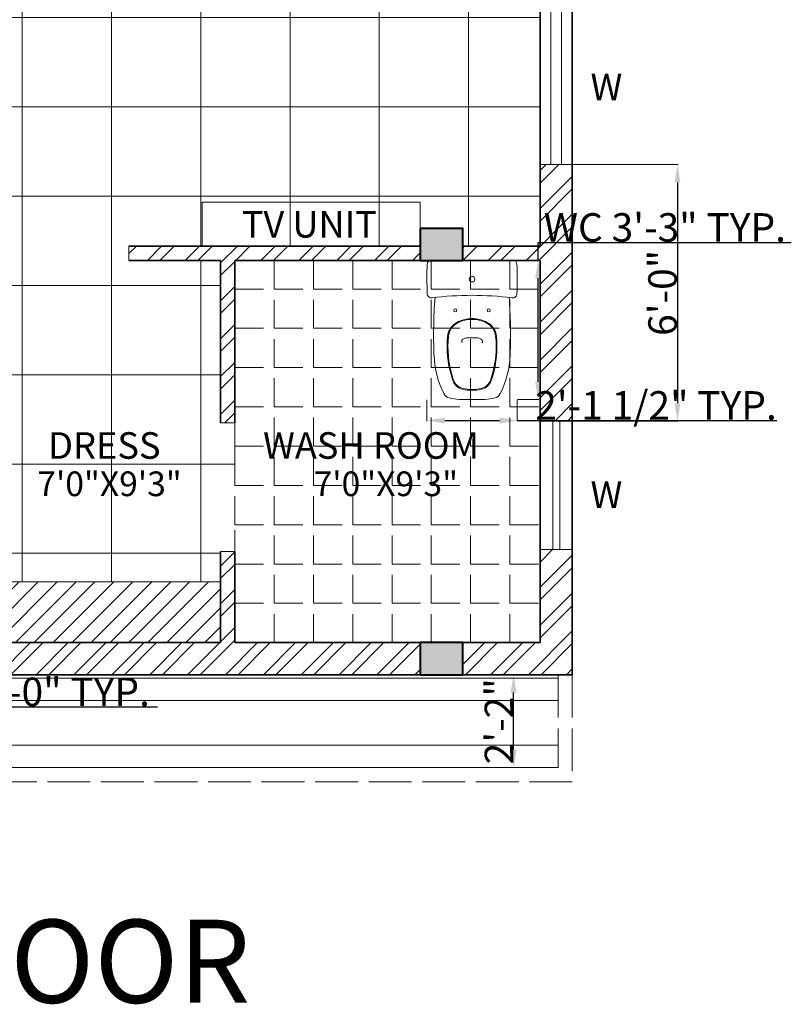
# Model space of a CAD drawing. Units: inches. Extents: x 351 to 1738, y -265 to 286.
# Tile 6 of 38: x 759 to 975, y -265 to 10. Entities that reach past the tile are written whole.
import ezdxf

# ---------------------------------------------------------------- set-up
doc = ezdxf.new("R2010")
doc.units = ezdxf.units.IN
doc.header["$MEASUREMENT"] = 0
doc.linetypes.add('ACAD_ISO02W100', pattern=[15, 12, -3])
doc.linetypes.add('ACAD_ISO03W100', pattern=[30, 12, -18])
for name, color, linetype, lineweight in [('A-ANNO-DIMS', 2, 'Continuous', 18), ('A-ANNO-SYMB', 7, 'Continuous', 18), ('A-ANNO-TEXT', 7, 'Continuous', 18), ('A-ANNO-TITL', 7, 'Continuous', 35), ('A-AREA-IDEN', 7, 'Continuous', 18), ('A-COLS', 7, 'Continuous', 40), ('A-COLS-PATT', 6, 'Continuous', 13), ('A-DOOR', 3, 'Continuous', 18), ('A-DOOR-HIDN', 3, 'ACAD_ISO03W100', 13), ('A-FLOR-CASE', 9, 'Continuous', 18), ('A-FLOR-CASE-PATT', 9, 'Continuous', 9), ('A-FLOR-FIXT', 9, 'Continuous', 18), ('A-FLOR-OVHD', 1, 'ACAD_ISO02W100', 18), ('A-FLOR-PATT', 9, 'Continuous', 9), ('A-GLAZ', 4, 'Continuous', 18), ('A-WALL', 7, 'Continuous', 35), ('A-WALL-PATT', 152, 'Continuous', 13)]:
    doc.layers.add(name, color=color, linetype=linetype, lineweight=lineweight)
doc.styles.add('Annotative', font='arial.ttf')
doc.styles.get("Standard").update_dxf_attribs({"font": 'arial.ttf'})
doc.dimstyles.get("Standard").update_dxf_attribs({"dimtxt": 8, "dimasz": 5, "dimexe": 0.18, "dimexo": 0.0625, "dimgap": 0.09, "dimtad": 1, "dimtoh": 1, "dimzin": 0, "dimdsep": 46, "dimlunit": 4, "dimtxsty": 'Standard', "dimcen": 0, "dimclre": 256, "dimadec": 0, "dimazin": 0, "dimtfac": 1, "dimtofl": 0, "dimtmove": 0, "dimatfit": 3, "dimfxl": 1, "dimtolj": 1, "dimtzin": 0, "dimlwe": -1, "dimarcsym": 0})

# ---------------------------------------------------------------- blocks, each defined once
blk = doc.blocks.new('A$C7E916B5A')
for p, q in [((0.019, 0.67), (0.2161, 0.67)), ((0.4133, 0.67), (0.2161, 0.67)), ((0.2161, 0.298), (0.1955, 0.298)), ((0.2161, 0.298), (0.2368, 0.298))]:
    blk.add_line(p, q)
for centre, radius in [((0.2161, 0.58), 0.0135), ((0.1361, 0.43), 0.0075), ((0.2961, 0.43), 0.0075)]:
    blk.add_circle(centre, radius)
for centre, radius, start, end in [((0.019, 0.651), 0.019, 90, 178.4999), ((0.4133, 0.651), 0.019, 1.5001, 90), ((2.5011, 0.586), 2.502, 178.4999, 181.7705), ((-2.0689, 0.586), 2.502, 358.2295, 1.5001), ((0.0203, 0.5093), 0.02, 181.7705, 277.4115), ((0.2161, -0.996), 1.498, 90, 97.4115), ((2.5311, 0.3098), 2.5, 175.7895, 182.2108), ((0.2161, -0.996), 1.498, 82.5885, 90), ((-2.0989, 0.3098), 2.5, 357.7892, 4.2105), ((0.412, 0.5093), 0.02, 262.5885, 358.2295), ((0.2161, 0.235), 0.155, 90, 118.1012), ((0.2161, 0.235), 0.151, 90, 118.1012), ((0.2161, 0.235), 0.155, 61.8988, 90), ((0.2161, 0.235), 0.151, 61.8988, 90), ((0.1832, 0.2967), 0.085, 118.1012, 174.3336), ((0.1832, 0.2967), 0.081, 118.1012, 174.3336), ((0.2491, 0.2967), 0.081, 5.6664, 61.8988), ((0.2491, 0.2967), 0.085, 5.6664, 61.8988), ((0.5961, 0.2558), 0.5, 174.3336, 196.4495), ((0.5961, 0.2558), 0.496, 174.3336, 196.4495), ((0.1781, 0.28), 0.012, 128.2132, 217.5723), ((0.1955, 0.258), 0.04, 90, 128.2132), ((0.2368, 0.258), 0.04, 51.7868, 90), ((0.2541, 0.28), 0.012, 322.4277, 51.7868), ((-0.1639, 0.2558), 0.496, 343.5505, 5.6664), ((-0.1639, 0.2558), 0.5, 343.5505, 5.6664), ((0.4827, 0.2307), 0.45, 182.2108, 206.6241), ((-0.0504, 0.2307), 0.45, 333.3759, 357.7892), ((0.4811, 0.2218), 0.38, 196.4495, 200.1007), ((0.4811, 0.2218), 0.376, 196.4495, 200.1007), ((-0.0488, 0.2218), 0.376, 339.8993, 343.5505), ((-0.0488, 0.2218), 0.38, 339.8993, 343.5505), ((0.1851, 0.1135), 0.0649, 200.1007, 256.7352), ((0.1851, 0.1135), 0.0609, 200.1007, 256.7352), ((0.2161, 0.245), 0.2, 256.7352, 270), ((0.2161, 0.245), 0.196, 256.7352, 270), ((0.2161, 0.245), 0.196, 270, 283.2648), ((0.2161, 0.245), 0.2, 270, 283.2648), ((0.2471, 0.1135), 0.0609, 283.2648, 339.8993), ((0.2471, 0.1135), 0.0649, 283.2648, 339.8993), ((0.1161, 0.047), 0.04, 206.6241, 256.4771), ((0.1652, 0.2512), 0.25, 256.477, 267.3481), ((0.2161, 1.35), 1.35, 267.3481, 270), ((0.2161, 1.35), 1.35, 270, 272.6519), ((0.267, 0.2512), 0.25, 272.6519, 283.523), ((0.3161, 0.047), 0.04, 283.5229, 333.3759)]:
    blk.add_arc(centre, radius, start, end)
blk = doc.blocks.new('*D5')
at = {"layer": 'A-ANNO-DIMS', "color": 0, "transparency": 16777216}
for p, q in [((910.09, -173.04), (897.53, -173.04)), ((910.09, -199.04), (897.53, -199.04))]:
    blk.add_line(p, q, dxfattribs=at)
at = {"layer": 'A-ANNO-DIMS', "color": 0, "lineweight": -2, "transparency": 16777216}
blk.add_line((897.71, -194.04), (897.71, -178.04), dxfattribs=at)
at = {"layer": 'A-ANNO-DIMS', "color": 0, "transparency": 16777216}
for points in [[(896.88, -178.04), (898.55, -178.04), (897.71, -173.04)], [(896.88, -194.04), (898.55, -194.04), (897.71, -199.04)]]:
    blk.add_solid(points, dxfattribs=at)
at = {"layer": 'Defpoints', "color": 0, "transparency": 16777216}
for p in [(897.71, -173.04), (910.16, -173.04), (910.16, -199.04)]:
    blk.add_point(p, dxfattribs=at)
at = {"layer": 'A-ANNO-DIMS', "color": 0, "transparency": 16777216, "insert": (893.61, -186.04), "char_height": 8, "attachment_point": 5, "rotation": 90}
blk.add_mtext('\\A1;2\'-2"', dxfattribs=at)
blk = doc.blocks.new('CONSOLE-TV')
blk.add_lwpolyline([(0, 0), (61, 0), (61, 12.29), (0, 12.29)], close=True)
blk = doc.blocks.new('COL-9x12')
blk.add_lwpolyline([(0, 12), (0, 0), (9, 0), (9, 12)], close=True)
blk = doc.blocks.new('WIN-36')
for p, q in [((0, 5.5), (36, 5.5)), ((0, 3.5), (36, 3.5))]:
    blk.add_line(p, q)
blk.add_lwpolyline([(0, 9), (36, 9), (36, 0), (0, 0)], close=True)
blk = doc.blocks.new('WIN-60')
for p, q in [((0, 6), (60, 6)), ((0, 3), (60, 3))]:
    blk.add_line(p, q)
blk.add_lwpolyline([(60, 0), (60, 9), (0, 9), (0, 0)], close=True)
blk = doc.blocks.new('*D34')
at = {"layer": 'A-ANNO-DIMS', "transparency": 16777216}
for p, q in [((631.58, -173.1), (631.58, -182.22)), ((691.58, -173.1), (691.58, -182.22))]:
    blk.add_line(p, q, dxfattribs=at)
at = {"layer": 'A-ANNO-DIMS', "color": 0, "lineweight": -2, "transparency": 16777216}
for p, q in [((636.58, -182.04), (686.58, -182.04)), ((691.58, -182.04), (797.99, -182.04))]:
    blk.add_line(p, q, dxfattribs=at)
at = {"layer": 'A-ANNO-DIMS', "color": 0, "transparency": 16777216}
for points in [[(636.58, -181.2), (636.58, -182.87), (631.58, -182.04)], [(686.58, -181.2), (686.58, -182.87), (691.58, -182.04)]]:
    blk.add_solid(points, dxfattribs=at)
at = {"layer": 'Defpoints', "color": 0, "transparency": 16777216}
for p in [(631.58, -173.04), (691.58, -173.04), (691.58, -182.04)]:
    blk.add_point(p, dxfattribs=at)
at = {"layer": 'A-ANNO-DIMS', "color": 0, "transparency": 16777216, "insert": (747.29, -177.81), "char_height": 8, "attachment_point": 5}
blk.add_mtext('\\A1;WINDOW 5\'-0" TYP.', dxfattribs=at)
blk = doc.blocks.new('*D44')
at = {"layer": 'A-ANNO-DIMS', "color": 0, "lineweight": -2, "transparency": 16777216}
for p, q in [((904.58, -57.01), (904.58, -52.01)), ((904.58, -52.01), (975.49, -52.01)), ((904.58, -91), (904.58, -62.01))]:
    blk.add_line(p, q, dxfattribs=at)
at = {"layer": 'A-ANNO-DIMS', "transparency": 16777216}
for p, q in [((898.79, -57.01), (904.76, -57.01)), ((898.79, -96), (904.76, -96))]:
    blk.add_line(p, q, dxfattribs=at)
at = {"layer": 'A-ANNO-DIMS', "color": 0, "transparency": 16777216}
for points in [[(903.75, -62.01), (905.41, -62.01), (904.58, -57.01)], [(903.75, -91), (905.41, -91), (904.58, -96)]]:
    blk.add_solid(points, dxfattribs=at)
at = {"layer": 'Defpoints', "color": 0, "transparency": 16777216}
for p in [(898.73, -57.01), (904.58, -57.01), (898.73, -96)]:
    blk.add_point(p, dxfattribs=at)
at = {"layer": 'A-ANNO-DIMS', "color": 0, "transparency": 16777216, "insert": (940.08, -47.78), "char_height": 8, "attachment_point": 5}
blk.add_mtext('\\A1;WC 3\'-3" TYP.', dxfattribs=at)
blk = doc.blocks.new('*D45')
at = {"layer": 'A-ANNO-DIMS', "transparency": 16777216}
for p, q in [((873.43, -96.06), (873.43, -102.03)), ((898.73, -96.06), (898.73, -102.03))]:
    blk.add_line(p, q, dxfattribs=at)
at = {"layer": 'A-ANNO-DIMS', "color": 0, "lineweight": -2, "transparency": 16777216}
for p, q in [((878.43, -101.85), (893.73, -101.85)), ((898.73, -101.85), (971.45, -101.85))]:
    blk.add_line(p, q, dxfattribs=at)
at = {"layer": 'A-ANNO-DIMS', "color": 0, "transparency": 16777216}
for points in [[(878.43, -101.02), (878.43, -102.68), (873.43, -101.85)], [(893.73, -101.02), (893.73, -102.68), (898.73, -101.85)]]:
    blk.add_solid(points, dxfattribs=at)
at = {"layer": 'Defpoints', "color": 0, "transparency": 16777216}
for p in [(873.43, -96), (898.73, -96), (898.73, -101.85)]:
    blk.add_point(p, dxfattribs=at)
at = {"layer": 'A-ANNO-DIMS', "color": 0, "transparency": 16777216, "insert": (937.59, -97.62), "char_height": 8, "attachment_point": 5}
blk.add_mtext('\\A1;2\'-1 1/2" TYP.', dxfattribs=at)
blk = doc.blocks.new('*D61')
at = {"layer": 'A-ANNO-DIMS', "transparency": 16777216}
for p, q in [((914.22, -30.19), (943.79, -30.19)), ((914.22, -102), (943.79, -102))]:
    blk.add_line(p, q, dxfattribs=at)
at = {"layer": 'A-ANNO-DIMS', "color": 0, "lineweight": -2, "transparency": 16777216}
blk.add_line((943.61, -35.19), (943.61, -97), dxfattribs=at)
at = {"layer": 'A-ANNO-DIMS', "color": 0, "transparency": 16777216}
for points in [[(942.77, -35.19), (944.44, -35.19), (943.61, -30.19)], [(942.77, -97), (944.44, -97), (943.61, -102)]]:
    blk.add_solid(points, dxfattribs=at)
at = {"layer": 'Defpoints', "color": 0, "transparency": 16777216}
for p in [(914.16, -30.19), (914.16, -102), (943.61, -102)]:
    blk.add_point(p, dxfattribs=at)
at = {"layer": 'A-ANNO-DIMS', "color": 0, "transparency": 16777216, "insert": (939.43, -66.09), "char_height": 8, "attachment_point": 5, "rotation": 90}
blk.add_mtext('\\A1;6\'-0"', dxfattribs=at)

msp = doc.modelspace()

# ---------------------------------------------------------------- hatches: boundary and pattern name
at = {"layer": 'A-COLS-PATT'}
h = msp.add_hatch(color=256, dxfattribs=at)
h.dxf.hatch_style = 1
h.paths.add_polyline_path([(460.155, 237.963), (451.155, 237.963), (451.155, 228.963), (460.155, 228.963)])
h.paths.add_polyline_path([(463.155, 237.963), (460.155, 237.963), (460.155, 228.963), (463.155, 228.963)])
h.paths.add_polyline_path([(391.155, 255.963), (382.155, 255.963), (382.155, 243.963), (391.155, 243.963)])
h.paths.add_polyline_path([(391.155, 210.963), (382.155, 210.963), (382.155, 198.963), (391.155, 198.963)])
h.paths.add_polyline_path([(391.155, -45.037), (382.155, -45.037), (382.155, -57.037), (391.155, -57.037)])
h.paths.add_polyline_path([(460.155, -45.037), (451.155, -45.037), (451.155, -57.037), (460.155, -57.037)])
h.paths.add_polyline_path([(460.155, -161.037), (451.155, -161.037), (451.155, -164.037), (451.155, -173.037), (460.155, -173.037)])
h.paths.add_polyline_path([(391.155, -161.037), (382.155, -161.037), (382.155, -173.037), (391.155, -173.037)])
h.paths.add_polyline_path([(596, -164.037), (584, -164.037), (584, -173.037), (596, -173.037)])
h.paths.add_polyline_path([(596, -50), (584, -50), (584, -59), (596, -59)])
h.paths.add_polyline_path([(596.155, 73.463), (592.155, 73.463), (592.155, 64.463), (596.155, 64.463)])
h.paths.add_polyline_path([(592.155, 73.463), (584.155, 73.463), (584.155, 64.463), (592.155, 64.463)])
h.paths.add_polyline_path([(596.155, 237.963), (584.155, 237.963), (584.155, 228.963), (596.155, 228.963)])
h.paths.add_polyline_path([(739.655, 237.963), (727.655, 237.963), (727.655, 228.963), (739.655, 228.963)])
h.paths.add_polyline_path([(883.515, 237.963), (871.515, 237.963), (871.515, 228.963), (883.515, 228.963)])
h.paths.add_polyline_path([(883.515, 73.463), (871.515, 73.463), (871.515, 64.463), (883.515, 64.463)])
h.paths.add_polyline_path([(731.655, 73.463), (727.655, 73.463), (727.655, 64.463), (731.655, 64.463)])
h.paths.add_polyline_path([(739.515, 73.463), (731.655, 73.463), (731.655, 64.463), (739.515, 64.463)])
h.paths.add_polyline_path([(883.515, -53.037), (871.515, -53.037), (871.515, -57.037), (883.515, -57.037)])
h.paths.add_polyline_path([(883.515, -48.037), (871.515, -48.037), (871.515, -53.037), (883.515, -53.037)])
h.paths.add_polyline_path([(739.515, -48.037), (727.515, -48.037), (727.515, -56.5), (727.516, -57.037), (739.515, -57.037)])
h.paths.add_polyline_path([(883.515, -164.037), (871.515, -164.037), (871.515, -173.037), (883.515, -173.037)])
at = {"layer": 'A-FLOR-CASE-PATT'}
h = msp.add_hatch(dxfattribs=at)
h.set_pattern_fill('ANSI31', color=256, scale=30)
h.set_pattern_definition([(45, (731.6553, -164.0373), (-2.65165, 2.65165), [])])
h.paths.add_polyline_path([(748.655, -57.037), (731.655, -57.037), (731.655, -164.037), (815.655, -164.037), (815.655, -147.037), (748.655, -147.037)])
at = {"layer": 'A-FLOR-PATT', "transparency": 33554559}
h = msp.add_hatch(dxfattribs=at)
h.set_pattern_fill('ANSI37', color=256, scale=200, angle=45)
h.set_pattern_definition([(90, (460.077, -164.037), (-25, 0), []), (180, (460.077, -164.037), (-4e-15, -25), [])])
h.paths.add_polyline_path([(727.516, -57.037), (727.515, -57.037), (727.515, -56.5), (727.5, -45), (727.5, -3.5), (727.501, -2.537), (725.797, -2.537), (725.797, -3.037), (721.988, -3.037), (721.988, -2.537), (717.916, -2.537), (717.916, -3.037), (714.106, -3.037), (714.106, -2.537), (710.487, -2.537), (710.487, -3.037), (706.677, -3.037), (706.677, -2.537), (702.965, -2.537), (702.965, -3.037), (699.155, -3.037), (699.155, -2.537), (694.965, -2.537), (694.965, -3.037), (691.155, -3.037), (691.155, -2.537), (679.655, -2.537), (678.797, -2.537), (677.776, -2.537), (676.723, -2.537), (652.655, -2.537), (651.799, -2.537), (650.778, -2.537), (649.725, -2.537), (625.877, -2.537), (624.879, -2.537), (623.857, -2.537), (622.804, -2.537), (596.155, -2.537), (596.155, -3.537), (460.155, -3.537), (460.155, -81.037), (460.077, -99.07), (460.077, -133.967), (460.155, -152.037), (460.155, -164.037), (485.277, -164.037), (545.277, -164.037), (727.655, -164.037)])
h.paths.add_polyline_path([(584, -59), (584, -50), (596, -50), (596, -59)], flags=16)
h.paths.add_polyline_path([(905.155, 204.963), (731.655, 204.963), (731.655, 73.463), (739.515, 73.463), (739.515, 64.463), (731.655, 64.463), (731.655, -3.5), (727.655, -3.5), (727.655, -3.537), (727.5, -45), (731.655, -45), (731.655, -48.037), (739.515, -48.037), (739.515, -53.037), (754, -53.037), (754, -57.037), (748.655, -57.037), (748.655, -147.037), (815.655, -147.037), (815.655, -138.5), (819.655, -138.5), (819.655, -102.5), (815.655, -102.5), (815.655, -57.037), (790, -57.037), (790, -53.037), (871.515, -53.037), (871.515, -48.037), (883.515, -48.037), (883.515, -53.037), (905.155, -53.037)])
h.paths.add_polyline_path([(871.515, 64.463), (871.515, 73.463), (883.515, 73.463), (883.515, 64.463)], flags=16)
h.paths.add_polyline_path([(727.655, 64.463), (685.515, 64.463), (685.515, 186.963), (638.155, 186.963), (638.155, 88.463), (596.155, 88.463), (596.155, 64.463), (584.155, 64.463), (584.155, 73.463), (592.155, 73.463), (592.155, 205.963), (574, 205.963), (574, 209.963), (538, 209.963), (538, 205.963), (536.5, 205.963), (536.5, 180), (489.5, 180), (489.5, 68.655), (460.155, 68.655), (460.155, 64.463), (536.155, 64.463), (536.155, 48.463), (532.155, 48.463), (532.155, 60.463), (460.155, 60.463), (460.155, 0.463), (532.155, 0.463), (532.155, 12.463), (536.155, 12.463), (536.155, 0.463), (596.155, 0.463), (596.155, -0.537), (622.655, -0.537), (623.655, -0.537), (624.655, -0.537), (625.655, -0.537), (649.655, -0.537), (650.576, -0.537), (651.576, -0.537), (652.576, -0.537), (676.655, -0.537), (677.574, -0.537), (678.574, -0.537), (679.574, -0.537), (691.155, -0.537), (691.155, -0.037), (694.965, -0.037), (694.965, -0.537), (699.155, -0.537), (699.155, -0.037), (702.965, -0.037), (702.965, -0.537), (706.677, -0.537), (706.677, -0.037), (710.487, -0.037), (710.487, -0.537), (714.106, -0.537), (714.106, -0.037), (717.916, -0.037), (717.916, -0.537), (721.988, -0.537), (721.988, -0.037), (725.797, -0.037), (725.797, -0.537), (727.655, -0.537)])
h.paths.add_polyline_path([(485.401, 6.538), (461.783, 6.538), (461.783, 51.327), (485.401, 51.327)], flags=16)
h.paths.add_polyline_path([(483.401, 8.538), (463.783, 8.538), (463.783, 49.327), (483.401, 49.327)], flags=0)
h.paths.add_polyline_path([(476.907, 30.5), (476.907, 29.5), (476.907, 26), (475.907, 26), (475.907, 29.5), (474.449, 29.5), (474.449, 26), (473.449, 26), (470.5, 26), (470.5, 27), (473.449, 27), (473.449, 29.5), (470.5, 29.5), (470.5, 32.758), (471.5, 32.758), (471.5, 30.5), (473.407, 30.5), (473.407, 32.897), (473.407, 33.897), (476.907, 33.897), (476.907, 32.897), (474.407, 32.897), (474.407, 30.5)], flags=0)
h = msp.add_hatch(dxfattribs=at)
h.set_pattern_fill('ANSI32', color=256, scale=50, angle=135)
h.set_pattern_definition([(180, (386.155, -199.037), (-2e-15, -18.75), []), (180, (379.905, -192.787), (-2e-15, -18.75), [])])
h.paths.add_polyline_path([(451.234, -133.967), (460.077, -133.967), (460.077, -99.07), (451.234, -99.07), (451.155, -81.037), (451.155, 98.963), (423.885, 98.963), (424, -81.037), (419, -81.037), (391.155, -81.037), (386.155, -81.037), (386.155, -161.037), (391.155, -161.037), (391.155, -173.037), (386.155, -173.037), (386.155, -199.037), (910.155, -199.037), (910.155, -173.037), (545.277, -173.037), (545.277, -164.037), (485.277, -164.037), (485.277, -173.037), (451.155, -173.037), (451.155, -161.037), (451.155, -152.037)])
at = {"layer": 'A-FLOR-PATT', "transparency": 33554610}
h = msp.add_hatch(dxfattribs=at)
h.set_pattern_fill('ANGLE', color=256, scale=40)
h.set_pattern_definition([(0, (819.655, -164.037), (0, 11), [8, -3]), (90, (819.655, -164.037), (-11, 7e-16), [8, -3])])
h.paths.add_polyline_path([(905.155, -57.037), (819.655, -57.037), (819.655, -102.5), (819.655, -138.5), (819.655, -164.037), (905.155, -164.037)])
at = {"layer": 'A-WALL-PATT'}
h = msp.add_hatch(dxfattribs=at)
h.set_pattern_fill('ANSI32', color=256, scale=20)
h.set_pattern_definition([(45, (382.155, -173.037), (-5.3033, 5.3033), []), (45, (385.691, -173.037), (-5.3033, 5.3033), [])])
h.paths.add_polyline_path([(391.155, -57.037), (382.155, -57.037), (382.155, -81.037), (391.155, -81.037)])
h.paths.add_polyline_path([(391.155, 198.963), (382.155, 198.963), (382.155, -45.037), (391.155, -45.037)])
h.paths.add_polyline_path([(391.155, 243.963), (382.155, 243.963), (382.155, 237.963), (382.155, 210.963), (391.155, 210.963)])
h.paths.add_polyline_path([(460.155, 255.963), (391.155, 255.963), (391.155, 246.963), (451.155, 246.963), (451.155, 237.963), (460.155, 237.963), (460.155, 251.963)])
h.paths.add_polyline_path([(404.155, 207.963), (391.155, 207.963), (391.155, 198.963), (404.155, 198.963)])
h.paths.add_polyline_path([(451.155, 207.963), (440.155, 207.963), (440.155, 198.963), (451.155, 198.963)])
h.paths.add_polyline_path([(460.155, 228.963), (451.155, 228.963), (451.155, 74.963), (460.155, 74.963), (460.155, 97.5)])
h.paths.add_polyline_path([(460.155, 60.463), (532.155, 60.463), (532.155, 48.463), (536.155, 48.463), (536.155, 64.463), (460.155, 64.463), (460.155, 62.963), (451.155, 62.963), (451.155, 46.258), (460.155, 46.258)])
h.paths.add_polyline_path([(460.155, -3.537), (596.155, -3.537), (596.155, 0.463), (536.155, 0.463), (536.155, 12.463), (532.155, 12.463), (532.155, 0.463), (460.155, 0.463), (460.155, 10.258), (451.155, 10.258), (451.155, -45.037), (460.155, -45.037)])
h.paths.add_polyline_path([(460.155, -57.037), (451.155, -57.037), (451.155, -81.037), (460.155, -81.037)])
h.paths.add_polyline_path([(460.155, -152.037), (451.155, -152.037), (451.155, -161.037), (460.155, -161.037)])
h.paths.add_polyline_path([(485.277, -164.037), (460.155, -164.037), (460.155, -164.5), (460.155, -173.037), (485.277, -173.037)])
h.paths.add_polyline_path([(584, -164.037), (545.277, -164.037), (545.277, -173.037), (584, -173.037)])
h.paths.add_polyline_path([(631.58, -164.037), (596, -164.037), (596, -173.037), (631.58, -173.037)])
h.paths.add_polyline_path([(871.515, -164.037), (819.655, -164.037), (819.655, -138.5), (815.655, -138.5), (815.655, -164.037), (691.58, -164.037), (691.58, -173.037), (871.515, -173.037)])
h.paths.add_polyline_path([(731.655, -57.037), (727.516, -57.037), (727.655, -164.037), (731.655, -164.037)])
h.paths.add_polyline_path([(914.155, -138), (905.155, -138), (905.155, -164.037), (883.515, -164.037), (883.515, -173.037), (914.155, -173.037)])
h.paths.add_polyline_path([(914.155, -30.189), (905.155, -30.189), (905.155, -53.037), (883.515, -53.037), (883.515, -57.037), (905.155, -57.037), (905.155, -102), (914.155, -102)])
h.paths.add_polyline_path([(871.515, -53.037), (790, -53.037), (790, -57.037), (815.655, -57.037), (815.655, -102.5), (819.655, -102.5), (819.655, -57.037), (871.515, -57.037)])
h.paths.add_polyline_path([(914.155, 120.993), (905.155, 120.993), (905.155, 29.811), (914.155, 29.811)])
h.paths.add_polyline_path([(731.655, 64.463), (727.655, 64.463), (727.655, -3.5), (731.655, -3.5)])
h.paths.add_polyline_path([(481.5, 209.963), (460.155, 209.963), (460.155, 205.963), (481.5, 205.963)])
h.paths.add_polyline_path([(538, 209.963), (517.5, 209.963), (517.5, 205.963), (538, 205.963)])
h.paths.add_polyline_path([(592.155, 209.963), (574, 209.963), (574, 205.963), (592.155, 205.963)])
h.paths.add_polyline_path([(596.155, 228.963), (592.155, 228.963), (592.155, 73.463), (596.155, 73.463)])
h.paths.add_polyline_path([(614, 237.963), (596.155, 237.963), (596.155, 228.963), (614, 228.963)])
h.paths.add_polyline_path([(677, 237.963), (650, 237.963), (650, 228.963), (677, 228.963)])
h.paths.add_polyline_path([(727.655, 237.963), (713, 237.963), (713, 228.963), (727.655, 228.963)])
h.paths.add_polyline_path([(871.515, 237.963), (739.655, 237.963), (739.655, 228.963), (871.515, 228.963)])
h.paths.add_polyline_path([(731.655, 228.963), (727.655, 228.963), (727.655, 73.463), (731.655, 73.463)])
h.paths.add_polyline_path([(914.155, 237.963), (883.515, 237.963), (883.515, 228.963), (905.155, 228.963), (905.155, 180.993), (914.155, 180.993)])

# ---------------------------------------------------------------- linework, layer by layer
at = {"layer": 'A-DOOR'}
for points in [[(790, -57.037), (790, -53.037)], [(819.655, -102.5), (815.655, -102.5)], [(815.655, -138.5), (819.655, -138.5)]]:
    msp.add_lwpolyline(points, dxfattribs=at)
at = {"layer": 'A-DOOR-HIDN'}
msp.add_line((819.655, -102.5), (819.655, -138.5), dxfattribs=at)
at = {"layer": 'A-FLOR-CASE'}
msp.add_line((748.655, -147.037), (815.655, -147.037), dxfattribs=at)
at = {"layer": 'A-FLOR-OVHD'}
for p, q in [((910.155, -173.037), (910.155, -199.037)), ((914.155, -173.037), (914.155, -203.037)), ((910.155, -199.037), (386.155, -199.037)), ((914.155, -203.037), (382.155, -203.037))]:
    msp.add_line(p, q, dxfattribs=at)
at = {"layer": 'A-WALL'}
for p, q in [((914.155, -173.037), (914.155, 237.963)), ((905.155, -53.037), (905.155, 228.963)), ((790, -53.037), (871.515, -53.037)), ((883.515, -53.037), (905.155, -53.037)), ((790, -57.037), (815.655, -57.037)), ((815.655, -57.037), (815.655, -102.5)), ((819.655, -57.037), (819.655, -102.5)), ((819.655, -57.037), (905.155, -57.037)), ((905.155, -164.037), (905.155, -57.037)), ((815.655, -138.5), (815.655, -164.037)), ((819.655, -138.5), (819.655, -164.037)), ((545.277, -164.037), (815.655, -164.037)), ((819.655, -164.037), (905.155, -164.037)), ((545.277, -173.037), (914.155, -173.037))]:
    msp.add_line(p, q, dxfattribs=at)

# ---------------------------------------------------------------- block references
at = {"layer": 'A-COLS'}
for p, rotation in [((883.515, -57.038), 90.00000000000007), ((883.515, -173.038), 90.00000000000018)]:
    msp.add_blockref('COL-9x12', p, dxfattribs=dict(at, rotation=rotation))
at = {"layer": 'A-FLOR-CASE'}
msp.add_blockref('CONSOLE-TV', (810.5, -53.037), dxfattribs=at)
at = {"layer": 'A-FLOR-FIXT', "xscale": 58.19959361425425, "yscale": 58.19959361425425, "zscale": 58.19959361425425}
msp.add_blockref('A$C7E916B5A', (873.5, -96), dxfattribs=at)
at = {"layer": 'A-GLAZ'}
for name, p, rotation in [('WIN-60', (914.155, -30.189), 90.00000000000003), ('WIN-36', (905.155, -102), 270.0000000000004)]:
    msp.add_blockref(name, p, dxfattribs=dict(at, rotation=rotation))

# ---------------------------------------------------------------- texts
at = {"layer": 'A-ANNO-SYMB', "style": 'Annotative'}
for p in [(919.256, -12.157), (919.256, -126.346)]:
    msp.add_text('W', height=7.433, dxfattribs=at).set_placement(p)
at = {"layer": 'A-ANNO-TEXT', "style": 'Annotative'}
msp.add_text('TV UNIT', height=7.4326, dxfattribs=at).set_placement((821.576, -50.615))
at = {"layer": 'A-ANNO-TITL', "style": 'Annotative'}
msp.add_text('DUPLEX SECOND FLOOR', height=23.27476, dxfattribs=at).set_placement((462.522, -264.89))
at = {"layer": 'A-AREA-IDEN', "style": 'Annotative'}
for s, height, p in [('DRESS', 7.4326, (767.365, -112.554)), ('WASH ROOM', 7.4326, (827.55, -112.554)), ('7\'0"X9\'3"', 6.9014, (764.321, -123.011)), ('7\'0"X9\'3"', 6.9014, (841.703, -123.011))]:
    msp.add_text(s, height=height, dxfattribs=at).set_placement(p)

# ---------------------------------------------------------------- dimensions: what is measured, and where the dimension line sits
at = {"layer": 'A-ANNO-DIMS'}
dim = msp.add_linear_dim(base=(904.58, -57.006), p1=(898.731, -96), p2=(898.731, -57.006), angle=90, text='WC <> TYP.', dimstyle='Standard', override={"dimdec": 1, "dimlfac": 1, "dimrnd": 0, "dimzin": 1, "dimdsep": 46, "dimlunit": 4, "dimfrac": 2}, dxfattribs=at)
dim.commit()
dim.dimension.update_dxf_attribs({"geometry": '*D44', "text_midpoint": (940.078, -47.777)})
for base, p1, p2, override, picture, middle in [((943.605, -102), (914.155, -30.189), (914.155, -102), {"dimdec": 1, "dimlfac": 1, "dimrnd": 0, "dimzin": 1, "dimdsep": 46, "dimlunit": 4, "dimfrac": 2}, '*D61', (939.431, -66.094)), ((897.714, -173.037), (910.155, -199.037), (910.155, -173.037), {"dimclrd": 0, "dimclre": 0, "dimclrt": 0}, '*D5', (893.608, -186.037))]:
    dim = msp.add_linear_dim(base=base, p1=p1, p2=p2, angle=90, dimstyle='Standard', override=override, dxfattribs=at)
    dim.commit()
    dim.dimension.update_dxf_attribs({"geometry": picture, "text_midpoint": middle})
for base, p1, p2, text, picture, middle in [((898.731, -101.849), (873.427, -96), (898.731, -96), '<> TYP.', '*D45', (937.592, -97.623)), ((691.58, -182.037), (631.58, -173.037), (691.58, -173.037), 'WINDOW <> TYP.', '*D34', (747.286, -177.808))]:
    dim = msp.add_linear_dim(base=base, p1=p1, p2=p2, text=text, dimstyle='Standard', override={"dimdec": 1, "dimlfac": 1, "dimrnd": 0, "dimzin": 1, "dimdsep": 46, "dimlunit": 4, "dimfrac": 2}, dxfattribs=at)
    dim.commit()
    dim.dimension.update_dxf_attribs({"geometry": picture, "text_midpoint": middle})

doc.saveas('drawing.dxf')
